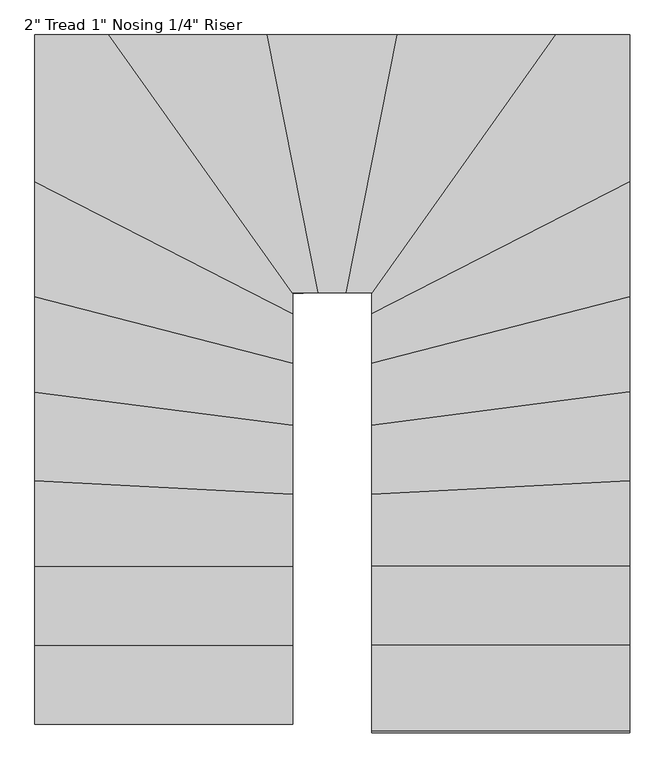
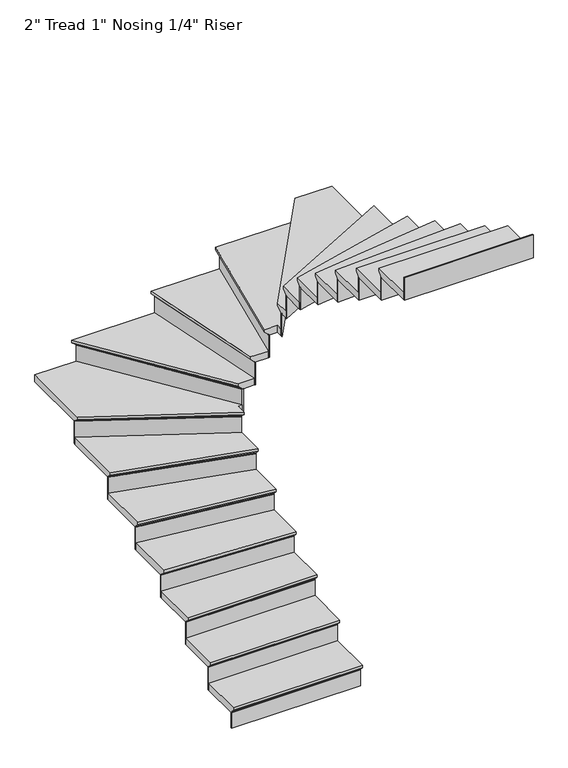
"""IFC4 building model written with IfcOpenShell, lengths in millimetres: stair flight geometry."""

from ifc_helpers import new_model, si_unit, origin, place, context, project, spatial, faceted_brep, source, transform, mapped, element, save


def stair_flight_9e59bd78(model_context):
    return source(origin(), model_context, "Body", "Brep", [
        faceted_brep([(-715.0890964, 3647.9718401, 150.2833333), (-715.0890964, 3647.9718401, 169.3333333), (-1629.4890964, 3647.9718401, 169.3333333), (-1629.4890964, 3647.9718401, 150.2833333), (-715.0890964, 3673.3718401, 124.8833333), (-1629.4890964, 3673.3718401, 124.8833333), (-715.0890964, 3952.7718401, 169.3333333), (-1629.4890964, 3952.7718401, 169.3333333), (-1629.4890964, 3673.3718401, 118.5333333), (-1629.4890964, 3952.7718401, 118.5333333), (-715.0890964, 3952.7718401, 118.5333333), (-715.0890964, 3673.3718401, 118.5333333)], [[[0, 1, 2, 3]], [[4, 0, 3, 5]], [[2, 1, 6, 7]], [[8, 9, 10, 11]], [[2, 7, 9, 8, 5, 3]], [[8, 11, 4, 5]], [[6, 1, 0, 4, 11, 10]], [[7, 6, 10, 9]]]),
        faceted_brep([(-715.0890964, 3673.3718401, 118.5333333), (-715.0890964, 3673.3718401, 0.0), (-715.0890964, 3679.7218401, 0.0), (-715.0890964, 3679.7218401, 118.5333333), (-1629.4890964, 3673.3718401, 118.5333333), (-1629.4890964, 3679.7218401, 118.5333333), (-1629.4890964, 3679.7218401, 0.0), (-1629.4890964, 3673.3718401, 0.0)], [[[0, 1, 2, 3]], [[4, 5, 6, 7]], [[1, 0, 4, 7]], [[2, 1, 7, 6]], [[3, 2, 6, 5]], [[0, 3, 5, 4]]]),
        faceted_brep([(-715.0890964, 3952.7718401, 287.8666667), (-715.0890964, 3952.7718401, 118.5333333), (-715.0890964, 3959.1218401, 118.5333333), (-715.0890964, 3959.1218401, 287.8666667), (-1629.4890964, 3952.7718401, 287.8666667), (-1629.4890964, 3959.1218401, 287.8666667), (-1629.4890964, 3959.1218401, 118.5333333), (-1629.4890964, 3952.7718401, 118.5333333)], [[[0, 1, 2, 3]], [[4, 5, 6, 7]], [[1, 0, 4, 7]], [[2, 1, 7, 6]], [[3, 2, 6, 5]], [[0, 3, 5, 4]]]),
        faceted_brep([(-1629.4890964, 3927.3718401, 338.6666667), (-715.0890964, 3927.3718401, 338.6666667), (-715.0890964, 4232.1718401, 338.6666667), (-1629.4890964, 4232.1718401, 338.6666667), (-1629.4890964, 3952.7718401, 287.8666667), (-1629.4890964, 4232.1718401, 287.8666667), (-715.0890964, 4232.1718401, 287.8666667), (-715.0890964, 3952.7718401, 287.8666667), (-1629.4890964, 3952.7718401, 294.2166667), (-1629.4890964, 3927.3718401, 319.6166667), (-715.0890964, 3952.7718401, 294.2166667), (-715.0890964, 3927.3718401, 319.6166667)], [[[0, 1, 2, 3]], [[4, 5, 6, 7]], [[0, 3, 5, 4, 8, 9]], [[4, 7, 10, 8]], [[2, 1, 11, 10, 7, 6]], [[3, 2, 6, 5]], [[11, 1, 0, 9]], [[10, 11, 9, 8]]]),
        faceted_brep([(-715.0890964, 4232.1718401, 457.2), (-715.0890964, 4232.1718401, 287.8666667), (-715.0890964, 4238.5218401, 287.8666667), (-715.0890964, 4238.5218401, 457.2), (-1629.4890964, 4232.1718401, 457.2), (-1629.4890964, 4238.5218401, 457.2), (-1629.4890964, 4238.5218401, 287.8666667), (-1629.4890964, 4232.1718401, 287.8666667)], [[[0, 1, 2, 3]], [[4, 5, 6, 7]], [[1, 0, 4, 7]], [[2, 1, 7, 6]], [[3, 2, 6, 5]], [[0, 3, 5, 4]]]),
        faceted_brep([(-1629.4890964, 4206.7718401, 508.0), (-715.0890964, 4206.7718401, 508.0), (-715.0890964, 4487.8390016, 508.0), (-1629.4890964, 4535.373272, 508.0), (-1629.4890964, 4232.1718401, 457.2), (-1629.4890964, 4535.373272, 457.2), (-715.0890964, 4487.8390016, 457.2), (-715.0890964, 4232.1718401, 457.2), (-1629.4890964, 4232.1718401, 463.55), (-1629.4890964, 4206.7718401, 488.95), (-715.0890964, 4232.1718401, 463.55), (-715.0890964, 4206.7718401, 488.95)], [[[0, 1, 2, 3]], [[4, 5, 6, 7]], [[0, 3, 5, 4, 8, 9]], [[4, 7, 10, 8]], [[2, 1, 11, 10, 7, 6]], [[3, 2, 6, 5]], [[11, 1, 0, 9]], [[10, 11, 9, 8]]]),
        faceted_brep([(-715.0890964, 4487.8390016, 626.5333333), (-715.0890964, 4487.8390016, 457.2), (-715.0890964, 4494.1975757, 457.2), (-715.0890964, 4494.1975757, 626.5333333), (-1629.4890964, 4535.373272, 626.5333333), (-1629.4890964, 4541.7318461, 626.5333333), (-1629.4890964, 4541.7318461, 457.2), (-1629.4890964, 4535.373272, 457.2)], [[[0, 1, 2, 3]], [[4, 5, 6, 7]], [[1, 0, 4, 7]], [[2, 1, 7, 6]], [[3, 2, 6, 5]], [[0, 3, 5, 4]]]),
        faceted_brep([(-1629.4890964, 4509.9389753, 677.3333333), (-715.0890964, 4462.4047049, 677.3333333), (-715.0890964, 4732.0057014, 677.3333333), (-1629.4890964, 4850.361753, 677.3333333), (-1629.4890964, 4535.373272, 626.5333333), (-1629.4890964, 4850.361753, 626.5333333), (-715.0890964, 4732.0057014, 626.5333333), (-715.0890964, 4487.8390016, 626.5333333), (-1629.4890964, 4535.373272, 632.8833333), (-1629.4890964, 4509.9389753, 658.2833333), (-715.0890964, 4487.8390016, 632.8833333), (-715.0890964, 4462.4047049, 658.2833333)], [[[0, 1, 2, 3]], [[4, 5, 6, 7]], [[0, 3, 5, 4, 8, 9]], [[4, 7, 10, 8]], [[2, 1, 11, 10, 7, 6]], [[3, 2, 6, 5]], [[11, 1, 0, 9]], [[10, 11, 9, 8]]]),
        faceted_brep([(-715.0890964, 4732.0057014, 795.8666667), (-715.0890964, 4732.0057014, 626.5333333), (-715.0890964, 4738.4086732, 626.5333333), (-715.0890964, 4738.4086732, 795.8666667), (-1629.4890964, 4850.361753, 795.8666667), (-1629.4890964, 4856.7647248, 795.8666667), (-1629.4890964, 4856.7647248, 626.5333333), (-1629.4890964, 4850.361753, 626.5333333)], [[[0, 1, 2, 3]], [[4, 5, 6, 7]], [[1, 0, 4, 7]], [[2, 1, 7, 6]], [[3, 2, 6, 5]], [[0, 3, 5, 4]]]),
        faceted_brep([(-1629.4890964, 4824.7498659, 846.6666667), (-715.0890964, 4706.3938143, 846.6666667), (-715.0890964, 4953.6329239, 846.6666667), (-1629.4890964, 5188.7633713, 846.6666667), (-1629.4890964, 4850.361753, 795.8666667), (-1629.4890964, 5188.7633713, 795.8666667), (-715.0890964, 4953.6329239, 795.8666667), (-715.0890964, 4732.0057014, 795.8666667), (-1629.4890964, 4850.361753, 802.2166667), (-1629.4890964, 4824.7498659, 827.6166667), (-715.0890964, 4732.0057014, 802.2166667), (-715.0890964, 4706.3938143, 827.6166667)], [[[0, 1, 2, 3]], [[4, 5, 6, 7]], [[0, 3, 5, 4, 8, 9]], [[4, 7, 10, 8]], [[2, 1, 11, 10, 7, 6]], [[3, 2, 6, 5]], [[11, 1, 0, 9]], [[10, 11, 9, 8]]]),
        faceted_brep([(-715.0890964, 4953.6329239, 965.2), (-715.0890964, 4953.6329239, 795.8666667), (-715.0890964, 4960.1895007, 795.8666667), (-715.0890964, 4960.1895007, 965.2), (-1629.4890964, 5188.7633713, 965.2), (-1629.4890964, 5195.3199481, 965.2), (-1629.4890964, 5195.3199481, 795.8666667), (-1629.4890964, 5188.7633713, 795.8666667)], [[[0, 1, 2, 3]], [[4, 5, 6, 7]], [[1, 0, 4, 7]], [[2, 1, 7, 6]], [[3, 2, 6, 5]], [[0, 3, 5, 4]]]),
        faceted_brep([(-1629.4890964, 5162.5370638, 1016.0), (-715.0890964, 4927.4066164, 1016.0), (-715.0890964, 5129.9795599, 1016.0), (-1629.4890964, 5598.8041813, 1016.0), (-1629.4890964, 5188.7633713, 965.2), (-1629.4890964, 5598.8041813, 965.2), (-715.0890964, 5129.9795599, 965.2), (-715.0890964, 4953.6329239, 965.2), (-1629.4890964, 5188.7633713, 971.55), (-1629.4890964, 5162.5370638, 996.95), (-715.0890964, 4953.6329239, 971.55), (-715.0890964, 4927.4066164, 996.95)], [[[0, 1, 2, 3]], [[4, 5, 6, 7]], [[0, 3, 5, 4, 8, 9]], [[4, 7, 10, 8]], [[2, 1, 11, 10, 7, 6]], [[3, 2, 6, 5]], [[11, 1, 0, 9]], [[10, 11, 9, 8]]]),
        faceted_brep([(-715.0890964, 5129.9795599, 1134.5333333), (-715.0890964, 5129.9795599, 965.2), (-715.0890964, 5137.1155431, 965.2), (-715.0890964, 5137.1155431, 1134.5333333), (-1629.4890964, 5598.8041813, 1134.5333333), (-1629.4890964, 5605.9401644, 1134.5333333), (-1629.4890964, 5605.9401644, 965.2), (-1629.4890964, 5598.8041813, 965.2)], [[[0, 1, 2, 3]], [[4, 5, 6, 7]], [[1, 0, 4, 7]], [[2, 1, 7, 6]], [[3, 2, 6, 5]], [[0, 3, 5, 4]]]),
        faceted_brep([(-1335.8079627, 6090.103532, 1185.3333333), (-1629.4890964, 6090.103532, 1185.3333333), (-1629.4890964, 5570.2602487, 1185.3333333), (-715.0890964, 5101.4356274, 1185.3333333), (-715.0890964, 5175.703532, 1185.3333333), (-685.5340135, 5175.703532, 1185.3333333), (-1629.4890964, 6090.103532, 1134.5333333), (-1335.8079627, 6090.103532, 1134.5333333), (-685.5340135, 5175.703532, 1134.5333333), (-715.0890964, 5175.703532, 1134.5333333), (-715.0890964, 5129.9795599, 1134.5333333), (-1629.4890964, 5598.8041813, 1134.5333333), (-1629.4890964, 5598.8041813, 1140.8833333), (-1629.4890964, 5570.2602487, 1166.2833333), (-715.0890964, 5129.9795599, 1140.8833333), (-715.0890964, 5101.4356274, 1166.2833333)], [[[0, 1, 2, 3, 4, 5]], [[6, 7, 8, 9, 10, 11]], [[1, 0, 7, 6]], [[2, 1, 6, 11, 12, 13]], [[11, 10, 14, 12]], [[4, 3, 15, 14, 10, 9]], [[5, 4, 9, 8]], [[0, 5, 8, 7]], [[15, 3, 2, 13]], [[14, 15, 13, 12]]]),
        faceted_brep([(-685.5340135, 5175.703532, 1303.8666667), (-685.5340135, 5175.703532, 1134.5333333), (-677.7420387, 5175.703532, 1134.5333333), (-677.7420387, 5175.703532, 1303.8666667), (-1335.8079627, 6090.103532, 1303.8666667), (-1328.0159879, 6090.103532, 1303.8666667), (-1328.0159879, 6090.103532, 1134.5333333), (-1335.8079627, 6090.103532, 1134.5333333)], [[[0, 1, 2, 3]], [[4, 5, 6, 7]], [[1, 0, 4, 7]], [[2, 1, 7, 6]], [[3, 2, 6, 5]], [[0, 3, 5, 4]]]),
        faceted_brep([(-1366.9758618, 6090.103532, 1354.6666667), (-716.7019127, 5175.703532, 1354.6666667), (-599.0799265, 5175.703532, 1354.6666667), (-779.3207828, 6090.103532, 1354.6666667), (-1335.8079627, 6090.103532, 1303.8666667), (-779.3207828, 6090.103532, 1303.8666667), (-599.0799265, 5175.703532, 1303.8666667), (-685.5340135, 5175.703532, 1303.8666667), (-1335.8079627, 6090.103532, 1310.2166667), (-1366.9758618, 6090.103532, 1335.6166667), (-685.5340135, 5175.703532, 1310.2166667), (-716.7019127, 5175.703532, 1335.6166667)], [[[0, 1, 2, 3]], [[4, 5, 6, 7]], [[0, 3, 5, 4, 8, 9]], [[4, 7, 10, 8]], [[2, 1, 11, 10, 7, 6]], [[3, 2, 6, 5]], [[11, 1, 0, 9]], [[10, 11, 9, 8]]]),
        faceted_brep([(-599.0799265, 5175.703532, 1473.2), (-599.0799265, 5175.703532, 1303.8666667), (-592.607741, 5175.703532, 1303.8666667), (-592.607741, 5175.703532, 1473.2), (-779.3207828, 6090.103532, 1473.2), (-772.8485973, 6090.103532, 1473.2), (-772.8485973, 6090.103532, 1303.8666667), (-779.3207828, 6090.103532, 1303.8666667)], [[[0, 1, 2, 3]], [[4, 5, 6, 7]], [[1, 0, 4, 7]], [[2, 1, 7, 6]], [[3, 2, 6, 5]], [[0, 3, 5, 4]]]),
        faceted_brep([(-805.2095245, 6090.103532, 1524.0), (-624.9686682, 5175.703532, 1524.0), (-499.9207828, 5175.703532, 1524.0), (-319.6799265, 6090.103532, 1524.0), (-779.3207828, 6090.103532, 1473.2), (-319.6799265, 6090.103532, 1473.2), (-499.9207828, 5175.703532, 1473.2), (-599.0799265, 5175.703532, 1473.2), (-779.3207828, 6090.103532, 1479.55), (-805.2095245, 6090.103532, 1504.95), (-599.0799265, 5175.703532, 1479.55), (-624.9686682, 5175.703532, 1504.95)], [[[0, 1, 2, 3]], [[4, 5, 6, 7]], [[0, 3, 5, 4, 8, 9]], [[4, 7, 10, 8]], [[2, 1, 11, 10, 7, 6]], [[3, 2, 6, 5]], [[11, 1, 0, 9]], [[10, 11, 9, 8]]]),
        faceted_brep([(-499.9207828, 5175.703532, 1642.5333333), (-499.9207828, 5175.703532, 1473.2), (-493.4485973, 5175.703532, 1473.2), (-493.4485973, 5175.703532, 1642.5333333), (-319.6799265, 6090.103532, 1642.5333333), (-313.207741, 6090.103532, 1642.5333333), (-313.207741, 6090.103532, 1473.2), (-319.6799265, 6090.103532, 1473.2)], [[[0, 1, 2, 3]], [[4, 5, 6, 7]], [[1, 0, 4, 7]], [[2, 1, 7, 6]], [[3, 2, 6, 5]], [[0, 3, 5, 4]]]),
        faceted_brep([(-345.5686682, 6090.103532, 1693.3333333), (-525.8095245, 5175.703532, 1693.3333333), (-435.6890964, 5175.703532, 1693.3333333), (-435.6890964, 5129.6080574, 1693.3333333), (247.3655683, 6090.103532, 1693.3333333), (-319.6799265, 6090.103532, 1642.5333333), (247.3655683, 6090.103532, 1642.5333333), (-435.6890964, 5129.6080574, 1642.5333333), (-435.6890964, 5175.703532, 1642.5333333), (-499.9207828, 5175.703532, 1642.5333333), (-319.6799265, 6090.103532, 1648.8833333), (-345.5686682, 6090.103532, 1674.2833333), (-499.9207828, 5175.703532, 1648.8833333), (-525.8095245, 5175.703532, 1674.2833333)], [[[0, 1, 2, 3, 4]], [[5, 6, 7, 8, 9]], [[0, 4, 6, 5, 10, 11]], [[5, 9, 12, 10]], [[2, 1, 13, 12, 9, 8]], [[3, 2, 8, 7]], [[4, 3, 7, 6]], [[13, 1, 0, 11]], [[12, 13, 11, 10]]]),
        faceted_brep([(-435.6890964, 5129.6080574, 1811.8666667), (-435.6890964, 5129.6080574, 1642.5333333), (-435.6890964, 5118.6511649, 1642.5333333), (-435.6890964, 5118.6511649, 1811.8666667), (247.3655683, 6090.103532, 1811.8666667), (255.1575431, 6090.103532, 1811.8666667), (255.1575431, 6090.103532, 1642.5333333), (247.3655683, 6090.103532, 1642.5333333)], [[[0, 1, 2, 3]], [[4, 5, 6, 7]], [[1, 0, 4, 7]], [[2, 1, 7, 6]], [[3, 2, 6, 5]], [[0, 3, 5, 4]]]),
        faceted_brep([(478.7109036, 5541.7163162, 1862.6666667), (478.7109036, 6090.103532, 1862.6666667), (216.1976691, 6090.103532, 1862.6666667), (-435.6890964, 5173.4356274, 1862.6666667), (-435.6890964, 5072.8916949, 1862.6666667), (478.7109036, 6090.103532, 1811.8666667), (478.7109036, 5541.7163162, 1811.8666667), (-435.6890964, 5072.8916949, 1811.8666667), (-435.6890964, 5129.6080574, 1811.8666667), (247.3655683, 6090.103532, 1811.8666667), (247.3655683, 6090.103532, 1818.2166667), (216.1976691, 6090.103532, 1843.6166667), (-435.6890964, 5129.6080574, 1818.2166667), (-435.6890964, 5173.4356274, 1843.6166667)], [[[0, 1, 2, 3, 4]], [[5, 6, 7, 8, 9]], [[1, 0, 6, 5]], [[2, 1, 5, 9, 10, 11]], [[9, 8, 12, 10]], [[4, 3, 13, 12, 8, 7]], [[0, 4, 7, 6]], [[13, 3, 2, 11]], [[12, 13, 11, 10]]]),
        faceted_brep([(-435.6890964, 5072.8916949, 1981.2), (-435.6890964, 5072.8916949, 1811.8666667), (-435.6890964, 5065.7557117, 1811.8666667), (-435.6890964, 5065.7557117, 1981.2), (478.7109036, 5541.7163162, 1981.2), (478.7109036, 5534.5803331, 1981.2), (478.7109036, 5534.5803331, 1811.8666667), (478.7109036, 5541.7163162, 1811.8666667)], [[[0, 1, 2, 3]], [[4, 5, 6, 7]], [[1, 0, 4, 7]], [[2, 1, 7, 6]], [[3, 2, 6, 5]], [[0, 3, 5, 4]]]),
        faceted_brep([(478.7109036, 5570.2602487, 2032.0), (-435.6890964, 5101.4356274, 2032.0), (-435.6890964, 4901.1803089, 2032.0), (478.7109036, 5136.3107563, 2032.0), (478.7109036, 5541.7163162, 1981.2), (478.7109036, 5136.3107563, 1981.2), (-435.6890964, 4901.1803089, 1981.2), (-435.6890964, 5072.8916949, 1981.2), (478.7109036, 5541.7163162, 1987.55), (478.7109036, 5570.2602487, 2012.95), (-435.6890964, 5072.8916949, 1987.55), (-435.6890964, 5101.4356274, 2012.95)], [[[0, 1, 2, 3]], [[4, 5, 6, 7]], [[0, 3, 5, 4, 8, 9]], [[4, 7, 10, 8]], [[2, 1, 11, 10, 7, 6]], [[3, 2, 6, 5]], [[11, 1, 0, 9]], [[10, 11, 9, 8]]]),
        faceted_brep([(-435.6890964, 4901.1803089, 2150.5333333), (-435.6890964, 4901.1803089, 1981.2), (-435.6890964, 4894.6237321, 1981.2), (-435.6890964, 4894.6237321, 2150.5333333), (478.7109036, 5136.3107563, 2150.5333333), (478.7109036, 5129.7541795, 2150.5333333), (478.7109036, 5129.7541795, 1981.2), (478.7109036, 5136.3107563, 1981.2)], [[[0, 1, 2, 3]], [[4, 5, 6, 7]], [[1, 0, 4, 7]], [[2, 1, 7, 6]], [[3, 2, 6, 5]], [[0, 3, 5, 4]]]),
        faceted_brep([(478.7109036, 5162.5370638, 2201.3333333), (-435.6890964, 4927.4066164, 2201.3333333), (-435.6890964, 4680.7819272, 2201.3333333), (478.7109036, 4799.1379788, 2201.3333333), (478.7109036, 5136.3107563, 2150.5333333), (478.7109036, 4799.1379788, 2150.5333333), (-435.6890964, 4680.7819272, 2150.5333333), (-435.6890964, 4901.1803089, 2150.5333333), (478.7109036, 5136.3107563, 2156.8833333), (478.7109036, 5162.5370638, 2182.2833333), (-435.6890964, 4901.1803089, 2156.8833333), (-435.6890964, 4927.4066164, 2182.2833333)], [[[0, 1, 2, 3]], [[4, 5, 6, 7]], [[0, 3, 5, 4, 8, 9]], [[4, 7, 10, 8]], [[2, 1, 11, 10, 7, 6]], [[3, 2, 6, 5]], [[11, 1, 0, 9]], [[10, 11, 9, 8]]]),
        faceted_brep([(-435.6890964, 4680.7819272, 2319.8666667), (-435.6890964, 4680.7819272, 2150.5333333), (-435.6890964, 4674.3789554, 2150.5333333), (-435.6890964, 4674.3789554, 2319.8666667), (478.7109036, 4799.1379788, 2319.8666667), (478.7109036, 4792.735007, 2319.8666667), (478.7109036, 4792.735007, 2150.5333333), (478.7109036, 4799.1379788, 2150.5333333)], [[[0, 1, 2, 3]], [[4, 5, 6, 7]], [[1, 0, 4, 7]], [[2, 1, 7, 6]], [[3, 2, 6, 5]], [[0, 3, 5, 4]]]),
        faceted_brep([(478.7109036, 4824.7498659, 2370.6666667), (-435.6890964, 4706.3938143, 2370.6666667), (-435.6890964, 4436.9704082, 2370.6666667), (478.7109036, 4484.5046786, 2370.6666667), (478.7109036, 4799.1379788, 2319.8666667), (478.7109036, 4484.5046786, 2319.8666667), (-435.6890964, 4436.9704082, 2319.8666667), (-435.6890964, 4680.7819272, 2319.8666667), (478.7109036, 4799.1379788, 2326.2166667), (478.7109036, 4824.7498659, 2351.6166667), (-435.6890964, 4680.7819272, 2326.2166667), (-435.6890964, 4706.3938143, 2351.6166667)], [[[0, 1, 2, 3]], [[4, 5, 6, 7]], [[0, 3, 5, 4, 8, 9]], [[4, 7, 10, 8]], [[2, 1, 11, 10, 7, 6]], [[3, 2, 6, 5]], [[11, 1, 0, 9]], [[10, 11, 9, 8]]]),
        faceted_brep([(-435.6890964, 4436.9704082, 2489.2), (-435.6890964, 4436.9704082, 2319.8666667), (-435.6890964, 4430.6118341, 2319.8666667), (-435.6890964, 4430.6118341, 2489.2), (478.7109036, 4484.5046786, 2489.2), (478.7109036, 4478.1461045, 2489.2), (478.7109036, 4478.1461045, 2319.8666667), (478.7109036, 4484.5046786, 2319.8666667)], [[[0, 1, 2, 3]], [[4, 5, 6, 7]], [[1, 0, 4, 7]], [[2, 1, 7, 6]], [[3, 2, 6, 5]], [[0, 3, 5, 4]]]),
        faceted_brep([(478.7109036, 4509.9389753, 2540.0), (-435.6890964, 4462.4047049, 2540.0), (-435.6890964, 4181.3718401, 2540.0), (478.7109036, 4181.3718401, 2540.0), (478.7109036, 4484.5046786, 2489.2), (478.7109036, 4181.3718401, 2489.2), (-435.6890964, 4181.3718401, 2489.2), (-435.6890964, 4436.9704082, 2489.2), (478.7109036, 4484.5046786, 2495.55), (478.7109036, 4509.9389753, 2520.95), (-435.6890964, 4436.9704082, 2495.55), (-435.6890964, 4462.4047049, 2520.95)], [[[0, 1, 2, 3]], [[4, 5, 6, 7]], [[0, 3, 5, 4, 8, 9]], [[4, 7, 10, 8]], [[2, 1, 11, 10, 7, 6]], [[3, 2, 6, 5]], [[11, 1, 0, 9]], [[10, 11, 9, 8]]]),
        faceted_brep([(-435.6890964, 4181.3718401, 2658.5333333), (-435.6890964, 4181.3718401, 2489.2), (-435.6890964, 4175.0218401, 2489.2), (-435.6890964, 4175.0218401, 2658.5333333), (478.7109036, 4181.3718401, 2658.5333333), (478.7109036, 4175.0218401, 2658.5333333), (478.7109036, 4175.0218401, 2489.2), (478.7109036, 4181.3718401, 2489.2)], [[[0, 1, 2, 3]], [[4, 5, 6, 7]], [[1, 0, 4, 7]], [[2, 1, 7, 6]], [[3, 2, 6, 5]], [[0, 3, 5, 4]]]),
        faceted_brep([(478.7109036, 4206.7718401, 2709.3333333), (-435.6890964, 4206.7718401, 2709.3333333), (-435.6890964, 3901.9718401, 2709.3333333), (478.7109036, 3901.9718401, 2709.3333333), (478.7109036, 4181.3718401, 2658.5333333), (478.7109036, 3901.9718401, 2658.5333333), (-435.6890964, 3901.9718401, 2658.5333333), (-435.6890964, 4181.3718401, 2658.5333333), (478.7109036, 4181.3718401, 2664.8833333), (478.7109036, 4206.7718401, 2690.2833333), (-435.6890964, 4181.3718401, 2664.8833333), (-435.6890964, 4206.7718401, 2690.2833333)], [[[0, 1, 2, 3]], [[4, 5, 6, 7]], [[0, 3, 5, 4, 8, 9]], [[4, 7, 10, 8]], [[2, 1, 11, 10, 7, 6]], [[3, 2, 6, 5]], [[11, 1, 0, 9]], [[10, 11, 9, 8]]]),
        faceted_brep([(-435.6890964, 3901.9718401, 2827.8666667), (-435.6890964, 3901.9718401, 2658.5333333), (-435.6890964, 3895.6218401, 2658.5333333), (-435.6890964, 3895.6218401, 2827.8666667), (478.7109036, 3901.9718401, 2827.8666667), (478.7109036, 3895.6218401, 2827.8666667), (478.7109036, 3895.6218401, 2658.5333333), (478.7109036, 3901.9718401, 2658.5333333)], [[[0, 1, 2, 3]], [[4, 5, 6, 7]], [[1, 0, 4, 7]], [[2, 1, 7, 6]], [[3, 2, 6, 5]], [[0, 3, 5, 4]]]),
        faceted_brep([(-435.6890964, 3622.5718401, 2997.2), (-435.6890964, 3622.5718401, 2827.8666667), (-435.6890964, 3616.2218401, 2827.8666667), (-435.6890964, 3616.2218401, 2997.2), (478.7109036, 3622.5718401, 2997.2), (478.7109036, 3616.2218401, 2997.2), (478.7109036, 3616.2218401, 2827.8666667), (478.7109036, 3622.5718401, 2827.8666667)], [[[0, 1, 2, 3]], [[4, 5, 6, 7]], [[1, 0, 4, 7]], [[2, 1, 7, 6]], [[3, 2, 6, 5]], [[0, 3, 5, 4]]]),
        faceted_brep([(478.7109036, 3927.3718401, 2878.6666667), (-435.6890964, 3927.3718401, 2878.6666667), (-435.6890964, 3622.5718401, 2878.6666667), (478.7109036, 3622.5718401, 2878.6666667), (478.7109036, 3901.9718401, 2827.8666667), (478.7109036, 3622.5718401, 2827.8666667), (-435.6890964, 3622.5718401, 2827.8666667), (-435.6890964, 3901.9718401, 2827.8666667), (478.7109036, 3901.9718401, 2834.2166667), (478.7109036, 3927.3718401, 2859.6166667), (-435.6890964, 3901.9718401, 2834.2166667), (-435.6890964, 3927.3718401, 2859.6166667)], [[[0, 1, 2, 3]], [[4, 5, 6, 7]], [[0, 3, 5, 4, 8, 9]], [[4, 7, 10, 8]], [[2, 1, 11, 10, 7, 6]], [[3, 2, 6, 5]], [[11, 1, 0, 9]], [[10, 11, 9, 8]]]),
    ])


if __name__ == "__main__":
    model = new_model("IFC4")
    model_context = context("Model", 3, world=origin())
    ifc_project = project(units=[si_unit("LENGTHUNIT", "METRE", prefix="MILLI")], contexts=[model_context])
    site = spatial("IfcSite", under=ifc_project)
    building = spatial("IfcBuilding", under=site)
    placement = place(None, origin())
    stair_flight_shape = stair_flight_9e59bd78(model_context)
    element("IfcStairFlight", 1, ObjectType="2\" Tread 1\" Nosing 1/4\" Riser", at=placement, inside=building, context=model_context, shape_type="MappedRepresentation", body=[
        mapped(stair_flight_shape, transform((0.0, 0.0, 0.0), x_axis=(1.0, 0.0, 0.0), y_axis=(0.0, 1.0, 0.0), z_axis=(0.0, 0.0, 1.0))),
    ])
    save(model, "model.ifc")
